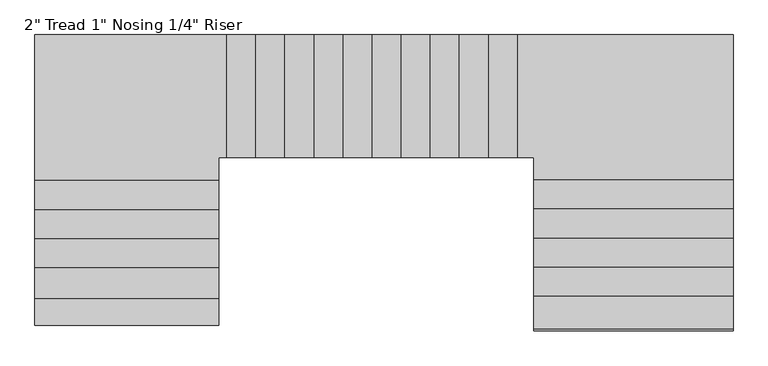
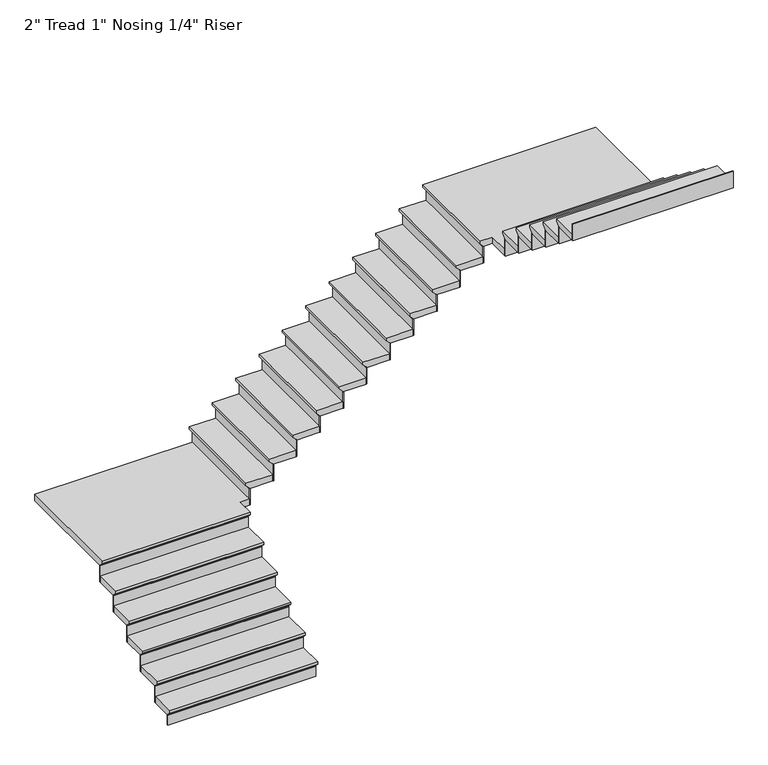
"""IFC4 building model written with IfcOpenShell, lengths in millimetres: stair flight geometry."""

from ifc_helpers import new_model, si_unit, origin, place, context, project, spatial, faceted_brep, source, transform, mapped, element, save


def stair_flight_e836c5a9(model_context):
    return source(origin(), model_context, "Body", "Brep", [
        faceted_brep([(-2368.6972892, 4718.9167606, 9714.6717391), (-2368.6972892, 4718.9167606, 9733.7217391), (-3493.0046642, 4718.9167606, 9733.7217391), (-3493.0046642, 4718.9167606, 9714.6717391), (-2368.6972892, 4744.3167606, 9689.2717391), (-3493.0046642, 4744.3167606, 9689.2717391), (-2368.6972892, 4909.4167606, 9733.7217391), (-3493.0046642, 4909.4167606, 9733.7217391), (-3493.0046642, 4744.3167606, 9682.9217391), (-3493.0046642, 4909.4167606, 9682.9217391), (-2368.6972892, 4909.4167606, 9682.9217391), (-2368.6972892, 4744.3167606, 9682.9217391)], [[[0, 1, 2, 3]], [[4, 0, 3, 5]], [[2, 1, 6, 7]], [[8, 9, 10, 11]], [[2, 7, 9, 8, 5, 3]], [[8, 11, 4, 5]], [[6, 1, 0, 4, 11, 10]], [[7, 6, 10, 9]]]),
        faceted_brep([(-2368.6972892, 4744.3167606, 9682.9217391), (-2368.6972892, 4744.3167606, 9601.2), (-2368.6972892, 4750.6667606, 9601.2), (-2368.6972892, 4750.6667606, 9682.9217391), (-3493.0046642, 4744.3167606, 9682.9217391), (-3493.0046642, 4750.6667606, 9682.9217391), (-3493.0046642, 4750.6667606, 9601.2), (-3493.0046642, 4744.3167606, 9601.2)], [[[0, 1, 2, 3]], [[4, 5, 6, 7]], [[1, 0, 4, 7]], [[2, 1, 7, 6]], [[3, 2, 6, 5]], [[0, 3, 5, 4]]]),
        faceted_brep([(-2368.6972892, 4909.4167606, 9815.4434783), (-2368.6972892, 4909.4167606, 9682.9217391), (-2368.6972892, 4915.7667606, 9682.9217391), (-2368.6972892, 4915.7667606, 9815.4434783), (-3493.0046642, 4909.4167606, 9815.4434783), (-3493.0046642, 4915.7667606, 9815.4434783), (-3493.0046642, 4915.7667606, 9682.9217391), (-3493.0046642, 4909.4167606, 9682.9217391)], [[[0, 1, 2, 3]], [[4, 5, 6, 7]], [[1, 0, 4, 7]], [[2, 1, 7, 6]], [[3, 2, 6, 5]], [[0, 3, 5, 4]]]),
        faceted_brep([(-3493.0046642, 4884.0167606, 9866.2434783), (-2368.6972892, 4884.0167606, 9866.2434783), (-2368.6972892, 5099.9164494, 9866.2434783), (-3493.0046642, 5099.9164494, 9866.2434783), (-3493.0046642, 4909.4167606, 9815.4434783), (-3493.0046642, 5099.9164494, 9815.4434783), (-2368.6972892, 5099.9164494, 9815.4434783), (-2368.6972892, 4909.4167606, 9815.4434783), (-3493.0046642, 4909.4167606, 9821.7934783), (-3493.0046642, 4884.0167606, 9847.1934783), (-2368.6972892, 4909.4167606, 9821.7934783), (-2368.6972892, 4884.0167606, 9847.1934783)], [[[0, 1, 2, 3]], [[4, 5, 6, 7]], [[0, 3, 5, 4, 8, 9]], [[4, 7, 10, 8]], [[2, 1, 11, 10, 7, 6]], [[3, 2, 6, 5]], [[11, 1, 0, 9]], [[10, 11, 9, 8]]]),
        faceted_brep([(-2368.6972892, 5099.9164494, 9947.9652174), (-2368.6972892, 5099.9164494, 9815.4434783), (-2368.6972892, 5106.2664494, 9815.4434783), (-2368.6972892, 5106.2664494, 9947.9652174), (-3493.0046642, 5099.9164494, 9947.9652174), (-3493.0046642, 5106.2664494, 9947.9652174), (-3493.0046642, 5106.2664494, 9815.4434783), (-3493.0046642, 5099.9164494, 9815.4434783)], [[[0, 1, 2, 3]], [[4, 5, 6, 7]], [[1, 0, 4, 7]], [[2, 1, 7, 6]], [[3, 2, 6, 5]], [[0, 3, 5, 4]]]),
        faceted_brep([(-3493.0046642, 5074.5164494, 9998.7652174), (-2368.6972892, 5074.5164494, 9998.7652174), (-2368.6972892, 5277.7164494, 9998.7652174), (-3493.0046642, 5277.7164494, 9998.7652174), (-3493.0046642, 5099.9164494, 9947.9652174), (-3493.0046642, 5277.7164494, 9947.9652174), (-2368.6972892, 5277.7164494, 9947.9652174), (-2368.6972892, 5099.9164494, 9947.9652174), (-3493.0046642, 5099.9164494, 9954.3152174), (-3493.0046642, 5074.5164494, 9979.7152174), (-2368.6972892, 5099.9164494, 9954.3152174), (-2368.6972892, 5074.5164494, 9979.7152174)], [[[0, 1, 2, 3]], [[4, 5, 6, 7]], [[0, 3, 5, 4, 8, 9]], [[4, 7, 10, 8]], [[2, 1, 11, 10, 7, 6]], [[3, 2, 6, 5]], [[11, 1, 0, 9]], [[10, 11, 9, 8]]]),
        faceted_brep([(-2368.6972892, 5277.7164494, 10080.4869565), (-2368.6972892, 5277.7164494, 9947.9652174), (-2368.6972892, 5284.0664494, 9947.9652174), (-2368.6972892, 5284.0664494, 10080.4869565), (-3493.0046642, 5277.7164494, 10080.4869565), (-3493.0046642, 5284.0664494, 10080.4869565), (-3493.0046642, 5284.0664494, 9947.9652174), (-3493.0046642, 5277.7164494, 9947.9652174)], [[[0, 1, 2, 3]], [[4, 5, 6, 7]], [[1, 0, 4, 7]], [[2, 1, 7, 6]], [[3, 2, 6, 5]], [[0, 3, 5, 4]]]),
        faceted_brep([(-3493.0046642, 5252.3164494, 10131.2869565), (-2368.6972892, 5252.3164494, 10131.2869565), (-2368.6972892, 5455.5164494, 10131.2869565), (-3493.0046642, 5455.5164494, 10131.2869565), (-3493.0046642, 5277.7164494, 10080.4869565), (-3493.0046642, 5455.5164494, 10080.4869565), (-2368.6972892, 5455.5164494, 10080.4869565), (-2368.6972892, 5277.7164494, 10080.4869565), (-3493.0046642, 5277.7164494, 10086.8369565), (-3493.0046642, 5252.3164494, 10112.2369565), (-2368.6972892, 5277.7164494, 10086.8369565), (-2368.6972892, 5252.3164494, 10112.2369565)], [[[0, 1, 2, 3]], [[4, 5, 6, 7]], [[0, 3, 5, 4, 8, 9]], [[4, 7, 10, 8]], [[2, 1, 11, 10, 7, 6]], [[3, 2, 6, 5]], [[11, 1, 0, 9]], [[10, 11, 9, 8]]]),
        faceted_brep([(-2368.6972892, 5455.5164494, 10213.0086957), (-2368.6972892, 5455.5164494, 10080.4869565), (-2368.6972892, 5461.8664494, 10080.4869565), (-2368.6972892, 5461.8664494, 10213.0086957), (-3493.0046642, 5455.5164494, 10213.0086957), (-3493.0046642, 5461.8664494, 10213.0086957), (-3493.0046642, 5461.8664494, 10080.4869565), (-3493.0046642, 5455.5164494, 10080.4869565)], [[[0, 1, 2, 3]], [[4, 5, 6, 7]], [[1, 0, 4, 7]], [[2, 1, 7, 6]], [[3, 2, 6, 5]], [[0, 3, 5, 4]]]),
        faceted_brep([(-3493.0046642, 5430.1164494, 10263.8086957), (-2368.6972892, 5430.1164494, 10263.8086957), (-2368.6972892, 5633.3167606, 10263.8086957), (-3493.0046642, 5633.3167606, 10263.8086957), (-3493.0046642, 5455.5164494, 10213.0086957), (-3493.0046642, 5633.3167606, 10213.0086957), (-2368.6972892, 5633.3167606, 10213.0086957), (-2368.6972892, 5455.5164494, 10213.0086957), (-3493.0046642, 5455.5164494, 10219.3586957), (-3493.0046642, 5430.1164494, 10244.7586957), (-2368.6972892, 5455.5164494, 10219.3586957), (-2368.6972892, 5430.1164494, 10244.7586957)], [[[0, 1, 2, 3]], [[4, 5, 6, 7]], [[0, 3, 5, 4, 8, 9]], [[4, 7, 10, 8]], [[2, 1, 11, 10, 7, 6]], [[3, 2, 6, 5]], [[11, 1, 0, 9]], [[10, 11, 9, 8]]]),
        faceted_brep([(-2368.6972892, 5633.3167606, 10345.5304348), (-2368.6972892, 5633.3167606, 10213.0086957), (-2368.6972892, 5639.6667606, 10213.0086957), (-2368.6972892, 5639.6667606, 10345.5304348), (-3493.0046642, 5633.3167606, 10345.5304348), (-3493.0046642, 5639.6667606, 10345.5304348), (-3493.0046642, 5639.6667606, 10213.0086957), (-3493.0046642, 5633.3167606, 10213.0086957)], [[[0, 1, 2, 3]], [[4, 5, 6, 7]], [[1, 0, 4, 7]], [[2, 1, 7, 6]], [[3, 2, 6, 5]], [[0, 3, 5, 4]]]),
        faceted_brep([(-2295.032382, 6496.9167606, 10396.3304348), (-3493.0046642, 6496.9167606, 10396.3304348), (-3493.0046642, 5607.9167606, 10396.3304348), (-2368.6972892, 5607.9167606, 10396.3304348), (-2368.6972892, 5746.5536537, 10396.3304348), (-2295.032382, 5746.5536537, 10396.3304348), (-3493.0046642, 6496.9167606, 10345.5304348), (-2295.032382, 6496.9167606, 10345.5304348), (-2295.032382, 5746.5536537, 10345.5304348), (-2368.6972892, 5746.5536537, 10345.5304348), (-2368.6972892, 5633.3167606, 10345.5304348), (-3493.0046642, 5633.3167606, 10345.5304348), (-3493.0046642, 5633.3167606, 10351.8804348), (-3493.0046642, 5607.9167606, 10377.2804348), (-2368.6972892, 5633.3167606, 10351.8804348), (-2368.6972892, 5607.9167606, 10377.2804348)], [[[0, 1, 2, 3, 4, 5]], [[6, 7, 8, 9, 10, 11]], [[1, 0, 7, 6]], [[2, 1, 6, 11, 12, 13]], [[11, 10, 14, 12]], [[4, 3, 15, 14, 10, 9]], [[5, 4, 9, 8]], [[0, 5, 8, 7]], [[15, 3, 2, 13]], [[14, 15, 13, 12]]]),
        faceted_brep([(-2295.032382, 5746.5536537, 10478.0521739), (-2295.032382, 5746.5536537, 10345.5304348), (-2288.682382, 5746.5536537, 10345.5304348), (-2288.682382, 5746.5536537, 10478.0521739), (-2295.032382, 6496.9167606, 10478.0521739), (-2288.682382, 6496.9167606, 10478.0521739), (-2288.682382, 6496.9167606, 10345.5304348), (-2295.032382, 6496.9167606, 10345.5304348)], [[[0, 1, 2, 3]], [[4, 5, 6, 7]], [[1, 0, 4, 7]], [[2, 1, 7, 6]], [[3, 2, 6, 5]], [[0, 3, 5, 4]]]),
        faceted_brep([(-2320.432382, 6496.9167606, 10528.8521739), (-2320.432382, 5746.5536537, 10528.8521739), (-2117.232382, 5746.5536537, 10528.8521739), (-2117.232382, 6496.9167606, 10528.8521739), (-2295.032382, 6496.9167606, 10478.0521739), (-2117.232382, 6496.9167606, 10478.0521739), (-2117.232382, 5746.5536537, 10478.0521739), (-2295.032382, 5746.5536537, 10478.0521739), (-2295.032382, 6496.9167606, 10484.4021739), (-2320.432382, 6496.9167606, 10509.8021739), (-2295.032382, 5746.5536537, 10484.4021739), (-2320.432382, 5746.5536537, 10509.8021739)], [[[0, 1, 2, 3]], [[4, 5, 6, 7]], [[0, 3, 5, 4, 8, 9]], [[4, 7, 10, 8]], [[2, 1, 11, 10, 7, 6]], [[3, 2, 6, 5]], [[11, 1, 0, 9]], [[10, 11, 9, 8]]]),
        faceted_brep([(-2117.232382, 5746.5536537, 10610.573913), (-2117.232382, 5746.5536537, 10478.0521739), (-2110.882382, 5746.5536537, 10478.0521739), (-2110.882382, 5746.5536537, 10610.573913), (-2117.232382, 6496.9167606, 10610.573913), (-2110.882382, 6496.9167606, 10610.573913), (-2110.882382, 6496.9167606, 10478.0521739), (-2117.232382, 6496.9167606, 10478.0521739)], [[[0, 1, 2, 3]], [[4, 5, 6, 7]], [[1, 0, 4, 7]], [[2, 1, 7, 6]], [[3, 2, 6, 5]], [[0, 3, 5, 4]]]),
        faceted_brep([(-2142.632382, 6496.9167606, 10661.373913), (-2142.632382, 5746.5536537, 10661.373913), (-1939.432382, 5746.5536537, 10661.373913), (-1939.432382, 6496.9167606, 10661.373913), (-2117.232382, 6496.9167606, 10610.573913), (-1939.432382, 6496.9167606, 10610.573913), (-1939.432382, 5746.5536537, 10610.573913), (-2117.232382, 5746.5536537, 10610.573913), (-2117.232382, 6496.9167606, 10616.923913), (-2142.632382, 6496.9167606, 10642.323913), (-2117.232382, 5746.5536537, 10616.923913), (-2142.632382, 5746.5536537, 10642.323913)], [[[0, 1, 2, 3]], [[4, 5, 6, 7]], [[0, 3, 5, 4, 8, 9]], [[4, 7, 10, 8]], [[2, 1, 11, 10, 7, 6]], [[3, 2, 6, 5]], [[11, 1, 0, 9]], [[10, 11, 9, 8]]]),
        faceted_brep([(-1939.432382, 5746.5536537, 10743.0956522), (-1939.432382, 5746.5536537, 10610.573913), (-1933.082382, 5746.5536537, 10610.573913), (-1933.082382, 5746.5536537, 10743.0956522), (-1939.432382, 6496.9167606, 10743.0956522), (-1933.082382, 6496.9167606, 10743.0956522), (-1933.082382, 6496.9167606, 10610.573913), (-1939.432382, 6496.9167606, 10610.573913)], [[[0, 1, 2, 3]], [[4, 5, 6, 7]], [[1, 0, 4, 7]], [[2, 1, 7, 6]], [[3, 2, 6, 5]], [[0, 3, 5, 4]]]),
        faceted_brep([(-1964.832382, 6496.9167606, 10793.8956522), (-1964.832382, 5746.5536537, 10793.8956522), (-1761.632382, 5746.5536537, 10793.8956522), (-1761.632382, 6496.9167606, 10793.8956522), (-1939.432382, 6496.9167606, 10743.0956522), (-1761.632382, 6496.9167606, 10743.0956522), (-1761.632382, 5746.5536537, 10743.0956522), (-1939.432382, 5746.5536537, 10743.0956522), (-1939.432382, 6496.9167606, 10749.4456522), (-1964.832382, 6496.9167606, 10774.8456522), (-1939.432382, 5746.5536537, 10749.4456522), (-1964.832382, 5746.5536537, 10774.8456522)], [[[0, 1, 2, 3]], [[4, 5, 6, 7]], [[0, 3, 5, 4, 8, 9]], [[4, 7, 10, 8]], [[2, 1, 11, 10, 7, 6]], [[3, 2, 6, 5]], [[11, 1, 0, 9]], [[10, 11, 9, 8]]]),
        faceted_brep([(-1761.632382, 5746.5536537, 10875.6173913), (-1761.632382, 5746.5536537, 10743.0956522), (-1755.282382, 5746.5536537, 10743.0956522), (-1755.282382, 5746.5536537, 10875.6173913), (-1761.632382, 6496.9167606, 10875.6173913), (-1755.282382, 6496.9167606, 10875.6173913), (-1755.282382, 6496.9167606, 10743.0956522), (-1761.632382, 6496.9167606, 10743.0956522)], [[[0, 1, 2, 3]], [[4, 5, 6, 7]], [[1, 0, 4, 7]], [[2, 1, 7, 6]], [[3, 2, 6, 5]], [[0, 3, 5, 4]]]),
        faceted_brep([(-1787.032382, 6496.9167606, 10926.4173913), (-1787.032382, 5746.5536537, 10926.4173913), (-1583.832382, 5746.5536537, 10926.4173913), (-1583.832382, 6496.9167606, 10926.4173913), (-1761.632382, 6496.9167606, 10875.6173913), (-1583.832382, 6496.9167606, 10875.6173913), (-1583.832382, 5746.5536537, 10875.6173913), (-1761.632382, 5746.5536537, 10875.6173913), (-1761.632382, 6496.9167606, 10881.9673913), (-1787.032382, 6496.9167606, 10907.3673913), (-1761.632382, 5746.5536537, 10881.9673913), (-1787.032382, 5746.5536537, 10907.3673913)], [[[0, 1, 2, 3]], [[4, 5, 6, 7]], [[0, 3, 5, 4, 8, 9]], [[4, 7, 10, 8]], [[2, 1, 11, 10, 7, 6]], [[3, 2, 6, 5]], [[11, 1, 0, 9]], [[10, 11, 9, 8]]]),
        faceted_brep([(-1583.832382, 5746.5536537, 11008.1391304), (-1583.832382, 5746.5536537, 10875.6173913), (-1577.482382, 5746.5536537, 10875.6173913), (-1577.482382, 5746.5536537, 11008.1391304), (-1583.832382, 6496.9167606, 11008.1391304), (-1577.482382, 6496.9167606, 11008.1391304), (-1577.482382, 6496.9167606, 10875.6173913), (-1583.832382, 6496.9167606, 10875.6173913)], [[[0, 1, 2, 3]], [[4, 5, 6, 7]], [[1, 0, 4, 7]], [[2, 1, 7, 6]], [[3, 2, 6, 5]], [[0, 3, 5, 4]]]),
        faceted_brep([(-1609.232382, 6496.9167606, 11058.9391304), (-1609.232382, 5746.5536537, 11058.9391304), (-1406.032382, 5746.5536537, 11058.9391304), (-1406.032382, 6496.9167606, 11058.9391304), (-1583.832382, 6496.9167606, 11008.1391304), (-1406.032382, 6496.9167606, 11008.1391304), (-1406.032382, 5746.5536537, 11008.1391304), (-1583.832382, 5746.5536537, 11008.1391304), (-1583.832382, 6496.9167606, 11014.4891304), (-1609.232382, 6496.9167606, 11039.8891304), (-1583.832382, 5746.5536537, 11014.4891304), (-1609.232382, 5746.5536537, 11039.8891304)], [[[0, 1, 2, 3]], [[4, 5, 6, 7]], [[0, 3, 5, 4, 8, 9]], [[4, 7, 10, 8]], [[2, 1, 11, 10, 7, 6]], [[3, 2, 6, 5]], [[11, 1, 0, 9]], [[10, 11, 9, 8]]]),
        faceted_brep([(-1406.032382, 5746.5536537, 11140.6608696), (-1406.032382, 5746.5536537, 11008.1391304), (-1399.682382, 5746.5536537, 11008.1391304), (-1399.682382, 5746.5536537, 11140.6608696), (-1406.032382, 6496.9167606, 11140.6608696), (-1399.682382, 6496.9167606, 11140.6608696), (-1399.682382, 6496.9167606, 11008.1391304), (-1406.032382, 6496.9167606, 11008.1391304)], [[[0, 1, 2, 3]], [[4, 5, 6, 7]], [[1, 0, 4, 7]], [[2, 1, 7, 6]], [[3, 2, 6, 5]], [[0, 3, 5, 4]]]),
        faceted_brep([(-1431.432382, 6496.9167606, 11191.4608696), (-1431.432382, 5746.5536537, 11191.4608696), (-1228.232382, 5746.5536537, 11191.4608696), (-1228.232382, 6496.9167606, 11191.4608696), (-1406.032382, 6496.9167606, 11140.6608696), (-1228.232382, 6496.9167606, 11140.6608696), (-1228.232382, 5746.5536537, 11140.6608696), (-1406.032382, 5746.5536537, 11140.6608696), (-1406.032382, 6496.9167606, 11147.0108696), (-1431.432382, 6496.9167606, 11172.4108696), (-1406.032382, 5746.5536537, 11147.0108696), (-1431.432382, 5746.5536537, 11172.4108696)], [[[0, 1, 2, 3]], [[4, 5, 6, 7]], [[0, 3, 5, 4, 8, 9]], [[4, 7, 10, 8]], [[2, 1, 11, 10, 7, 6]], [[3, 2, 6, 5]], [[11, 1, 0, 9]], [[10, 11, 9, 8]]]),
        faceted_brep([(-1228.232382, 5746.5536537, 11273.1826087), (-1228.232382, 5746.5536537, 11140.6608696), (-1221.882382, 5746.5536537, 11140.6608696), (-1221.882382, 5746.5536537, 11273.1826087), (-1228.232382, 6496.9167606, 11273.1826087), (-1221.882382, 6496.9167606, 11273.1826087), (-1221.882382, 6496.9167606, 11140.6608696), (-1228.232382, 6496.9167606, 11140.6608696)], [[[0, 1, 2, 3]], [[4, 5, 6, 7]], [[1, 0, 4, 7]], [[2, 1, 7, 6]], [[3, 2, 6, 5]], [[0, 3, 5, 4]]]),
        faceted_brep([(-1253.632382, 6496.9167606, 11323.9826087), (-1253.632382, 5746.5536537, 11323.9826087), (-1050.432382, 5746.5536537, 11323.9826087), (-1050.432382, 6496.9167606, 11323.9826087), (-1228.232382, 6496.9167606, 11273.1826087), (-1050.432382, 6496.9167606, 11273.1826087), (-1050.432382, 5746.5536537, 11273.1826087), (-1228.232382, 5746.5536537, 11273.1826087), (-1228.232382, 6496.9167606, 11279.5326087), (-1253.632382, 6496.9167606, 11304.9326087), (-1228.232382, 5746.5536537, 11279.5326087), (-1253.632382, 5746.5536537, 11304.9326087)], [[[0, 1, 2, 3]], [[4, 5, 6, 7]], [[0, 3, 5, 4, 8, 9]], [[4, 7, 10, 8]], [[2, 1, 11, 10, 7, 6]], [[3, 2, 6, 5]], [[11, 1, 0, 9]], [[10, 11, 9, 8]]]),
        faceted_brep([(-1050.432382, 5746.5536537, 11405.7043478), (-1050.432382, 5746.5536537, 11273.1826087), (-1044.082382, 5746.5536537, 11273.1826087), (-1044.082382, 5746.5536537, 11405.7043478), (-1050.432382, 6496.9167606, 11405.7043478), (-1044.082382, 6496.9167606, 11405.7043478), (-1044.082382, 6496.9167606, 11273.1826087), (-1050.432382, 6496.9167606, 11273.1826087)], [[[0, 1, 2, 3]], [[4, 5, 6, 7]], [[1, 0, 4, 7]], [[2, 1, 7, 6]], [[3, 2, 6, 5]], [[0, 3, 5, 4]]]),
        faceted_brep([(-1075.832382, 6496.9167606, 11456.5043478), (-1075.832382, 5746.5536537, 11456.5043478), (-872.632382, 5746.5536537, 11456.5043478), (-872.632382, 6496.9167606, 11456.5043478), (-1050.432382, 6496.9167606, 11405.7043478), (-872.632382, 6496.9167606, 11405.7043478), (-872.632382, 5746.5536537, 11405.7043478), (-1050.432382, 5746.5536537, 11405.7043478), (-1050.432382, 6496.9167606, 11412.0543478), (-1075.832382, 6496.9167606, 11437.4543478), (-1050.432382, 5746.5536537, 11412.0543478), (-1075.832382, 5746.5536537, 11437.4543478)], [[[0, 1, 2, 3]], [[4, 5, 6, 7]], [[0, 3, 5, 4, 8, 9]], [[4, 7, 10, 8]], [[2, 1, 11, 10, 7, 6]], [[3, 2, 6, 5]], [[11, 1, 0, 9]], [[10, 11, 9, 8]]]),
        faceted_brep([(-872.632382, 5746.5536537, 11538.226087), (-872.632382, 5746.5536537, 11405.7043478), (-866.282382, 5746.5536537, 11405.7043478), (-866.282382, 5746.5536537, 11538.226087), (-872.632382, 6496.9167606, 11538.226087), (-866.282382, 6496.9167606, 11538.226087), (-866.282382, 6496.9167606, 11405.7043478), (-872.632382, 6496.9167606, 11405.7043478)], [[[0, 1, 2, 3]], [[4, 5, 6, 7]], [[1, 0, 4, 7]], [[2, 1, 7, 6]], [[3, 2, 6, 5]], [[0, 3, 5, 4]]]),
        faceted_brep([(-898.032382, 6496.9167606, 11589.026087), (-898.032382, 5746.5536537, 11589.026087), (-694.832382, 5746.5536537, 11589.026087), (-694.832382, 6496.9167606, 11589.026087), (-872.632382, 6496.9167606, 11538.226087), (-694.832382, 6496.9167606, 11538.226087), (-694.832382, 5746.5536537, 11538.226087), (-872.632382, 5746.5536537, 11538.226087), (-872.632382, 6496.9167606, 11544.576087), (-898.032382, 6496.9167606, 11569.976087), (-872.632382, 5746.5536537, 11544.576087), (-898.032382, 5746.5536537, 11569.976087)], [[[0, 1, 2, 3]], [[4, 5, 6, 7]], [[0, 3, 5, 4, 8, 9]], [[4, 7, 10, 8]], [[2, 1, 11, 10, 7, 6]], [[3, 2, 6, 5]], [[11, 1, 0, 9]], [[10, 11, 9, 8]]]),
        faceted_brep([(-694.832382, 5746.5536537, 11670.7478261), (-694.832382, 5746.5536537, 11538.226087), (-688.482382, 5746.5536537, 11538.226087), (-688.482382, 5746.5536537, 11670.7478261), (-694.832382, 6496.9167606, 11670.7478261), (-688.482382, 6496.9167606, 11670.7478261), (-688.482382, 6496.9167606, 11538.226087), (-694.832382, 6496.9167606, 11538.226087)], [[[0, 1, 2, 3]], [[4, 5, 6, 7]], [[1, 0, 4, 7]], [[2, 1, 7, 6]], [[3, 2, 6, 5]], [[0, 3, 5, 4]]]),
        faceted_brep([(-720.232382, 6496.9167606, 11721.5478261), (-720.232382, 5746.5536537, 11721.5478261), (-517.032382, 5746.5536537, 11721.5478261), (-517.032382, 6496.9167606, 11721.5478261), (-694.832382, 6496.9167606, 11670.7478261), (-517.032382, 6496.9167606, 11670.7478261), (-517.032382, 5746.5536537, 11670.7478261), (-694.832382, 5746.5536537, 11670.7478261), (-694.832382, 6496.9167606, 11677.0978261), (-720.232382, 6496.9167606, 11702.4978261), (-694.832382, 5746.5536537, 11677.0978261), (-720.232382, 5746.5536537, 11702.4978261)], [[[0, 1, 2, 3]], [[4, 5, 6, 7]], [[0, 3, 5, 4, 8, 9]], [[4, 7, 10, 8]], [[2, 1, 11, 10, 7, 6]], [[3, 2, 6, 5]], [[11, 1, 0, 9]], [[10, 11, 9, 8]]]),
        faceted_brep([(-517.032382, 5746.5536537, 11803.2695652), (-517.032382, 5746.5536537, 11670.7478261), (-510.682382, 5746.5536537, 11670.7478261), (-510.682382, 5746.5536537, 11803.2695652), (-517.032382, 6496.9167606, 11803.2695652), (-510.682382, 6496.9167606, 11803.2695652), (-510.682382, 6496.9167606, 11670.7478261), (-517.032382, 6496.9167606, 11670.7478261)], [[[0, 1, 2, 3]], [[4, 5, 6, 7]], [[1, 0, 4, 7]], [[2, 1, 7, 6]], [[3, 2, 6, 5]], [[0, 3, 5, 4]]]),
        faceted_brep([(774.1953358, 5582.5167606, 11854.0695652), (774.1953358, 6496.9167606, 11854.0695652), (-542.432382, 6496.9167606, 11854.0695652), (-542.432382, 5746.5536537, 11854.0695652), (-445.0046642, 5746.5536537, 11854.0695652), (-445.0046642, 5582.5167606, 11854.0695652), (774.1953358, 6496.9167606, 11803.2695652), (774.1953358, 5582.5167606, 11803.2695652), (-445.0046642, 5582.5167606, 11803.2695652), (-445.0046642, 5746.5536537, 11803.2695652), (-517.032382, 5746.5536537, 11803.2695652), (-517.032382, 6496.9167606, 11803.2695652), (-517.032382, 6496.9167606, 11809.6195652), (-542.432382, 6496.9167606, 11835.0195652), (-517.032382, 5746.5536537, 11809.6195652), (-542.432382, 5746.5536537, 11835.0195652)], [[[0, 1, 2, 3, 4, 5]], [[6, 7, 8, 9, 10, 11]], [[1, 0, 7, 6]], [[2, 1, 6, 11, 12, 13]], [[11, 10, 14, 12]], [[4, 3, 15, 14, 10, 9]], [[5, 4, 9, 8]], [[0, 5, 8, 7]], [[15, 3, 2, 13]], [[14, 15, 13, 12]]]),
        faceted_brep([(-445.0046642, 5582.5167606, 11935.7913043), (-445.0046642, 5582.5167606, 11803.2695652), (-445.0046642, 5576.1667606, 11803.2695652), (-445.0046642, 5576.1667606, 11935.7913043), (774.1953358, 5582.5167606, 11935.7913043), (774.1953358, 5576.1667606, 11935.7913043), (774.1953358, 5576.1667606, 11803.2695652), (774.1953358, 5582.5167606, 11803.2695652)], [[[0, 1, 2, 3]], [[4, 5, 6, 7]], [[1, 0, 4, 7]], [[2, 1, 7, 6]], [[3, 2, 6, 5]], [[0, 3, 5, 4]]]),
        faceted_brep([(774.1953358, 5607.9167606, 11986.5913043), (-445.0046642, 5607.9167606, 11986.5913043), (-445.0046642, 5404.7164494, 11986.5913043), (774.1953358, 5404.7164494, 11986.5913043), (774.1953358, 5582.5167606, 11935.7913043), (774.1953358, 5404.7164494, 11935.7913043), (-445.0046642, 5404.7164494, 11935.7913043), (-445.0046642, 5582.5167606, 11935.7913043), (774.1953358, 5582.5167606, 11942.1413043), (774.1953358, 5607.9167606, 11967.5413043), (-445.0046642, 5582.5167606, 11942.1413043), (-445.0046642, 5607.9167606, 11967.5413043)], [[[0, 1, 2, 3]], [[4, 5, 6, 7]], [[0, 3, 5, 4, 8, 9]], [[4, 7, 10, 8]], [[2, 1, 11, 10, 7, 6]], [[3, 2, 6, 5]], [[11, 1, 0, 9]], [[10, 11, 9, 8]]]),
        faceted_brep([(-445.0046642, 5404.7164494, 12068.3130435), (-445.0046642, 5404.7164494, 11935.7913043), (-445.0046642, 5398.3664494, 11935.7913043), (-445.0046642, 5398.3664494, 12068.3130435), (774.1953358, 5404.7164494, 12068.3130435), (774.1953358, 5398.3664494, 12068.3130435), (774.1953358, 5398.3664494, 11935.7913043), (774.1953358, 5404.7164494, 11935.7913043)], [[[0, 1, 2, 3]], [[4, 5, 6, 7]], [[1, 0, 4, 7]], [[2, 1, 7, 6]], [[3, 2, 6, 5]], [[0, 3, 5, 4]]]),
        faceted_brep([(774.1953358, 5430.1164494, 12119.1130435), (-445.0046642, 5430.1164494, 12119.1130435), (-445.0046642, 5226.9164494, 12119.1130435), (774.1953358, 5226.9164494, 12119.1130435), (774.1953358, 5404.7164494, 12068.3130435), (774.1953358, 5226.9164494, 12068.3130435), (-445.0046642, 5226.9164494, 12068.3130435), (-445.0046642, 5404.7164494, 12068.3130435), (774.1953358, 5404.7164494, 12074.6630435), (774.1953358, 5430.1164494, 12100.0630435), (-445.0046642, 5404.7164494, 12074.6630435), (-445.0046642, 5430.1164494, 12100.0630435)], [[[0, 1, 2, 3]], [[4, 5, 6, 7]], [[0, 3, 5, 4, 8, 9]], [[4, 7, 10, 8]], [[2, 1, 11, 10, 7, 6]], [[3, 2, 6, 5]], [[11, 1, 0, 9]], [[10, 11, 9, 8]]]),
        faceted_brep([(-445.0046642, 5226.9164494, 12200.8347826), (-445.0046642, 5226.9164494, 12068.3130435), (-445.0046642, 5220.5664494, 12068.3130435), (-445.0046642, 5220.5664494, 12200.8347826), (774.1953358, 5226.9164494, 12200.8347826), (774.1953358, 5220.5664494, 12200.8347826), (774.1953358, 5220.5664494, 12068.3130435), (774.1953358, 5226.9164494, 12068.3130435)], [[[0, 1, 2, 3]], [[4, 5, 6, 7]], [[1, 0, 4, 7]], [[2, 1, 7, 6]], [[3, 2, 6, 5]], [[0, 3, 5, 4]]]),
        faceted_brep([(774.1953358, 5252.3164494, 12251.6347826), (-445.0046642, 5252.3164494, 12251.6347826), (-445.0046642, 5049.1164494, 12251.6347826), (774.1953358, 5049.1164494, 12251.6347826), (774.1953358, 5226.9164494, 12200.8347826), (774.1953358, 5049.1164494, 12200.8347826), (-445.0046642, 5049.1164494, 12200.8347826), (-445.0046642, 5226.9164494, 12200.8347826), (774.1953358, 5226.9164494, 12207.1847826), (774.1953358, 5252.3164494, 12232.5847826), (-445.0046642, 5226.9164494, 12207.1847826), (-445.0046642, 5252.3164494, 12232.5847826)], [[[0, 1, 2, 3]], [[4, 5, 6, 7]], [[0, 3, 5, 4, 8, 9]], [[4, 7, 10, 8]], [[2, 1, 11, 10, 7, 6]], [[3, 2, 6, 5]], [[11, 1, 0, 9]], [[10, 11, 9, 8]]]),
        faceted_brep([(-445.0046642, 5049.1164494, 12333.3565217), (-445.0046642, 5049.1164494, 12200.8347826), (-445.0046642, 5042.7664494, 12200.8347826), (-445.0046642, 5042.7664494, 12333.3565217), (774.1953358, 5049.1164494, 12333.3565217), (774.1953358, 5042.7664494, 12333.3565217), (774.1953358, 5042.7664494, 12200.8347826), (774.1953358, 5049.1164494, 12200.8347826)], [[[0, 1, 2, 3]], [[4, 5, 6, 7]], [[1, 0, 4, 7]], [[2, 1, 7, 6]], [[3, 2, 6, 5]], [[0, 3, 5, 4]]]),
        faceted_brep([(774.1953358, 5074.5164494, 12384.1565217), (-445.0046642, 5074.5164494, 12384.1565217), (-445.0046642, 4871.3164494, 12384.1565217), (774.1953358, 4871.3164494, 12384.1565217), (774.1953358, 5049.1164494, 12333.3565217), (774.1953358, 4871.3164494, 12333.3565217), (-445.0046642, 4871.3164494, 12333.3565217), (-445.0046642, 5049.1164494, 12333.3565217), (774.1953358, 5049.1164494, 12339.7065217), (774.1953358, 5074.5164494, 12365.1065217), (-445.0046642, 5049.1164494, 12339.7065217), (-445.0046642, 5074.5164494, 12365.1065217)], [[[0, 1, 2, 3]], [[4, 5, 6, 7]], [[0, 3, 5, 4, 8, 9]], [[4, 7, 10, 8]], [[2, 1, 11, 10, 7, 6]], [[3, 2, 6, 5]], [[11, 1, 0, 9]], [[10, 11, 9, 8]]]),
        faceted_brep([(-445.0046642, 4871.3164494, 12465.8782609), (-445.0046642, 4871.3164494, 12333.3565217), (-445.0046642, 4864.9664494, 12333.3565217), (-445.0046642, 4864.9664494, 12465.8782609), (774.1953358, 4871.3164494, 12465.8782609), (774.1953358, 4864.9664494, 12465.8782609), (774.1953358, 4864.9664494, 12333.3565217), (774.1953358, 4871.3164494, 12333.3565217)], [[[0, 1, 2, 3]], [[4, 5, 6, 7]], [[1, 0, 4, 7]], [[2, 1, 7, 6]], [[3, 2, 6, 5]], [[0, 3, 5, 4]]]),
        faceted_brep([(-445.0046642, 4693.5167606, 12598.4), (-445.0046642, 4693.5167606, 12465.8782609), (-445.0046642, 4687.1667606, 12465.8782609), (-445.0046642, 4687.1667606, 12598.4), (774.1953358, 4693.5167606, 12598.4), (774.1953358, 4687.1667606, 12598.4), (774.1953358, 4687.1667606, 12465.8782609), (774.1953358, 4693.5167606, 12465.8782609)], [[[0, 1, 2, 3]], [[4, 5, 6, 7]], [[1, 0, 4, 7]], [[2, 1, 7, 6]], [[3, 2, 6, 5]], [[0, 3, 5, 4]]]),
        faceted_brep([(774.1953358, 4896.7164494, 12516.6782609), (-445.0046642, 4896.7164494, 12516.6782609), (-445.0046642, 4693.5167606, 12516.6782609), (774.1953358, 4693.5167606, 12516.6782609), (774.1953358, 4871.3164494, 12465.8782609), (774.1953358, 4693.5167606, 12465.8782609), (-445.0046642, 4693.5167606, 12465.8782609), (-445.0046642, 4871.3164494, 12465.8782609), (774.1953358, 4871.3164494, 12472.2282609), (774.1953358, 4896.7164494, 12497.6282609), (-445.0046642, 4871.3164494, 12472.2282609), (-445.0046642, 4896.7164494, 12497.6282609)], [[[0, 1, 2, 3]], [[4, 5, 6, 7]], [[0, 3, 5, 4, 8, 9]], [[4, 7, 10, 8]], [[2, 1, 11, 10, 7, 6]], [[3, 2, 6, 5]], [[11, 1, 0, 9]], [[10, 11, 9, 8]]]),
    ])


if __name__ == "__main__":
    model = new_model("IFC4")
    model_context = context("Model", 3, world=origin())
    ifc_project = project(units=[si_unit("LENGTHUNIT", "METRE", prefix="MILLI")], contexts=[model_context])
    site = spatial("IfcSite", under=ifc_project)
    building = spatial("IfcBuilding", under=site)
    placement = place(None, origin())
    stair_flight_shape = stair_flight_e836c5a9(model_context)
    element("IfcStairFlight", 1, ObjectType="2\" Tread 1\" Nosing 1/4\" Riser", at=placement, inside=building, context=model_context, shape_type="MappedRepresentation", body=[
        mapped(stair_flight_shape, transform((0.0, 0.0, 0.0), x_axis=(1.0, 0.0, 0.0), y_axis=(0.0, 1.0, 0.0), z_axis=(0.0, 0.0, 1.0))),
    ])
    save(model, "model.ifc")
